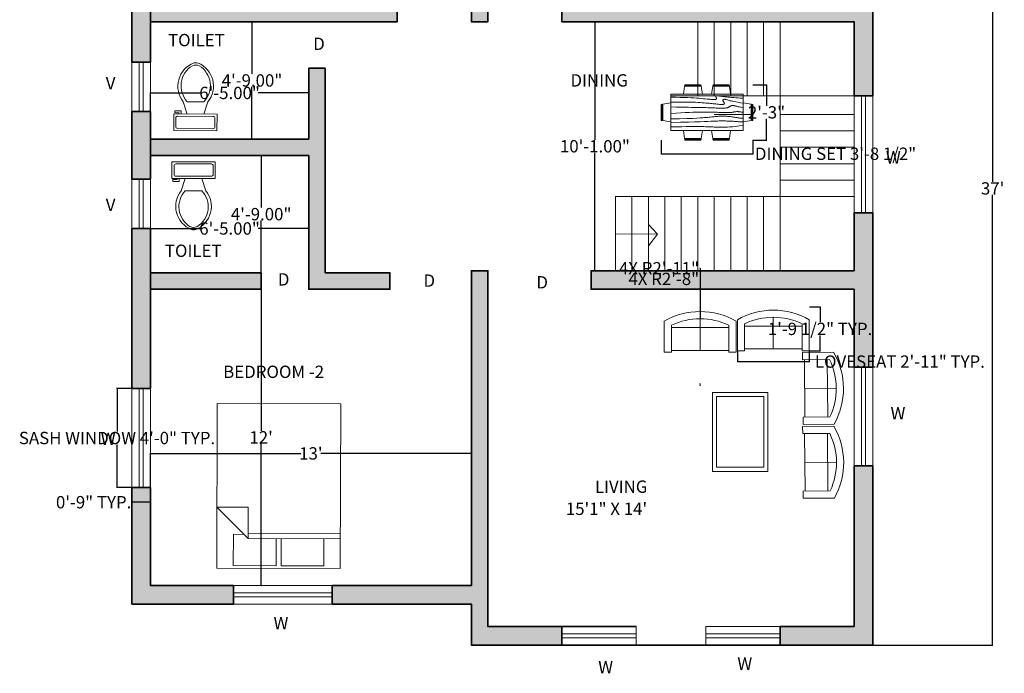
# Model space of a CAD drawing. Units: inches. Extents: x -977 to 1065, y -406 to 125.
# Tile 3 of 4: x 571 to 1049, y -406 to -89. Entities that reach past the tile are written whole.
import ezdxf

# ---------------------------------------------------------------- set-up
doc = ezdxf.new("R2010")
doc.units = ezdxf.units.IN
doc.header["$MEASUREMENT"] = 0
for name, color, linetype, lineweight in [('A-ANNO-DIMS', 2, 'Continuous', 13), ('A-ANNO-TEXT', 7, 'Continuous', 18), ('A-AREA-IDEN', 7, 'Continuous', 18), ('A-FLOR-FIXT', 8, 'Continuous', 18), ('A-FLOR-STRS', 7, 'Continuous', 18), ('A-FURN', 8, 'Continuous', 18), ('A-GLAZ', 5, 'Continuous', 18), ('A-WALL', 7, 'Continuous', 35), ('A-WALL-PATT', 252, 'Continuous', 13)]:
    doc.layers.add(name, color=color, linetype=linetype, lineweight=lineweight)
doc.styles.get("Standard").update_dxf_attribs({"font": 'arial.ttf'})
doc.dimstyles.get("Standard").update_dxf_attribs({"dimtxt": 6, "dimasz": 0.18, "dimexe": 0.18, "dimexo": 0.0625, "dimgap": 0.09, "dimtad": 0, "dimtih": 1, "dimtoh": 1, "dimzin": 0, "dimdsep": 46, "dimlunit": 3, "dimtxsty": 'Standard', "dimcen": 0.09, "dimadec": 0, "dimazin": 0, "dimtfac": 1, "dimtofl": 0, "dimtmove": 0, "dimatfit": 3, "dimfxl": 1, "dimtolj": 1, "dimtzin": 0, "dimarcsym": 0})

# ---------------------------------------------------------------- blocks, each defined once
blk = doc.blocks.new('Sofa - Roundback Loveseat 5 ft.')
for p, q in [((0, -32.44198), (0, -5.99998)), ((-24, -33.99998), (-24, -11.46958)), ((-23.9998, -13.38178), (23.99986, -13.38178)), ((24.00004, -33.99998), (24.00004, -11.46958)), ((-24, -32.44198), (24.00004, -32.44198))]:
    blk.add_line(p, q)
for points in [[(-24, -33.99998), (-30, -33.99998), (-30, -7.99998)], [(30.00004, -7.99998), (30.00004, -33.99998), (24.00004, -33.99998)]]:
    blk.add_lwpolyline(points)
for centre, radius, start, end in [((0, -60.24998), 60.24998, 60.13715, 119.8628), ((0, -61.38438), 55.38444, 64.32083, 115.6792)]:
    blk.add_arc(centre, radius, start, end)
blk = doc.blocks.new('*U27')
for p, q in [((9.5, -6), (9.5, -2)), ((-10, -8.5), (-8, -8.5)), ((-10, -9.5), (-10, -8.5)), ((-7, -9.5), (-10, -9.5)), ((-8, -8.5), (-8, -8)), ((-7, -8), (-7, -9.5)), ((-4, -8), (-6, -14)), ((4, -8), (6, -14)), ((4, -14), (-4, -14))]:
    blk.add_line(p, q)
blk.add_lwpolyline([(10.5, -8), (10.5, 0), (-10.5, 0), (-10.5, -8)], close=True)
for points in [[(-9.5, -2), (-9.5, -6)], [(8.5, -1), (-8.5, -1)], [(-8.5, -7), (8.5, -7)]]:
    blk.add_lwpolyline(points)
for centre, radius, start, end in [((-8.62, -1.88), 0.884, 81.8699, 188.1301), ((8.62, -1.88), 0.884, 351.8699, 98.1301), ((-8.62, -6.12), 0.884, 171.8699, 278.1301), ((8.62, -6.12), 0.884, 261.8699, 8.1301), ((3.52, -21.58), 12.17, 141.4691, 247.9714), ((4.2, -21.82), 11.33, 136.3677, 238.9468), ((-3.52, -21.58), 12.17, 292.0284, 38.5307), ((-4.2, -21.82), 11.33, 301.053, 43.6321), ((0, -27.88), 4, 245.7318, 294.2682), ((0, -29), 4, 254.8605, 285.1395)]:
    blk.add_arc(centre, radius, start, end)
blk = doc.blocks.new('Dining Set - 36 x 72 in.')
for p, q in [((-22.2343, 26.00059), (-23.4847, 17.99762)), ((-22.2304, 26), (-5.7608, 26)), ((-22, 27.5), (-22.1562, 26.50042)), ((-5.8416, 26.5), (-22.1534, 26.5)), ((-22, 27.5), (-6, 27.5)), ((-5.8437, 26.49966), (-6, 27.5)), ((-4.5152, 17.99762), (-5.7655, 25.99926)), ((5.7657, 26.00059), (4.5153, 17.99762)), ((5.7696, 26), (22.2392, 26)), ((6, 27.5), (5.8438, 26.50042)), ((22.1584, 26.5), (5.8466, 26.5)), ((6, 27.5), (22, 27.5)), ((22.1563, 26.49966), (22, 27.5)), ((23.4848, 17.99762), (22.2345, 25.99926)), ((36, 18), (-36, 18)), ((-36, 18), (-36, -18)), ((36, -18), (36, 18)), ((-45.5, 8), (-44.5004, 8.15617)), ((-45.5, 8), (-45.5, -8)), ((-44.5, -8.15843), (-44.5, 8.15338)), ((-44.0006, 8.23428), (-35.9976, 9.48474)), ((-44, 8.23041), (-44, -8.23915)), ((44.0006, 8.23428), (35.9976, 9.48474)), ((44, 8.23041), (44, -8.23915)), ((44.5, -8.15843), (44.5, 8.15338)), ((45.5, 8), (44.5005, 8.15617)), ((45.5, 8), (45.5, -8)), ((-44.4997, -8.15631), (-45.5, -8)), ((-35.9976, -9.48476), (-43.9993, -8.2345)), ((35.9976, -9.48476), (43.9993, -8.2345)), ((44.4997, -8.15631), (45.5, -8)), ((-36, -18), (36, -18)), ((-22.2343, -26.0006), (-23.4847, -17.99762)), ((-4.5152, -17.99762), (-5.7655, -25.99928)), ((5.7657, -26.0006), (4.5153, -17.99762)), ((23.4848, -17.99762), (22.2345, -25.99928)), ((-22.2304, -26), (-5.7608, -26)), ((-22, -27.5), (-22.1562, -26.50044)), ((-5.8416, -26.5), (-22.1534, -26.5)), ((-22, -27.5), (-6, -27.5)), ((-5.8437, -26.49967), (-6, -27.5)), ((5.7696, -26), (22.2392, -26)), ((6, -27.5), (5.8438, -26.50044)), ((22.1584, -26.5), (5.8466, -26.5)), ((6, -27.5), (22, -27.5)), ((22.1563, -26.49967), (22, -27.5))]:
    blk.add_line(p, q)
for points in [[(-36, 15), (-31.1772, 14.97754), (-26.8079, 14.91406), (-22.8538, 14.81543), (-19.276, 14.6875), (-16.0362, 14.53613), (-13.0957, 14.36718), (-10.4159, 14.18652), (-7.9583, 14), (-5.6904, 13.81315), (-3.6035, 13.63021), (-1.6954, 13.45508), (0.0365, 13.29166), (1.5945, 13.14388), (2.9811, 13.01562), (4.1988, 12.9108), (5.25, 12.83333), (6.1393, 12.78613), (6.8802, 12.76823), (7.4883, 12.77767), (7.9792, 12.8125), (8.3685, 12.87077), (8.6719, 12.95052), (8.9049, 13.0498), (9.0833, 13.16666), (9.2205, 13.29899), (9.3216, 13.44401), (9.3895, 13.59879), (9.4271, 13.76041), (9.4373, 13.92594), (9.4232, 14.09245), (9.3875, 14.257), (9.3333, 14.41666), (9.2638, 14.56917), (9.1836, 14.71484), (9.0975, 14.85465), (9.0104, 14.98958), (8.9272, 15.1206), (8.8529, 15.2487), (8.7922, 15.37483), (8.75, 15.5), (8.7305, 15.62467), (8.7344, 15.74739), (8.7617, 15.86621), (8.8125, 15.97916), (8.8867, 16.08431), (8.9844, 16.17968), (9.1055, 16.26334), (9.25, 16.33333), (9.4189, 16.38802), (9.6172, 16.42708), (9.8506, 16.45052), (10.125, 16.45833), (10.4463, 16.45052), (10.8203, 16.42708), (11.2529, 16.38802), (11.75, 16.33333), (12.3184, 16.26318), (12.9694, 16.17838), (13.7151, 16.07991), (14.5677, 15.96875), (15.5395, 15.84586), (16.6426, 15.71224), (17.8893, 15.56884), (19.2917, 15.41666), (20.859, 15.25667), (22.5879, 15.08984), (24.4721, 14.91715), (26.5052, 14.73958), (28.6809, 14.5581), (30.9929, 14.3737), (33.4347, 14.18733), (36, 14)], [(-36, 10), (-28.9766, 10.14274), (-23.1725, 10.20442), (-18.4241, 10.19775), (-14.5677, 10.13541), (-11.4399, 10.03011), (-8.877, 9.89453), (-6.7154, 9.74137), (-4.7917, 9.58333), (-2.9698, 9.43082), (-1.2246, 9.28515), (0.4415, 9.14534), (2.026, 9.01041), (3.5266, 8.87939), (4.9408, 8.7513), (6.266, 8.62516), (7.5, 8.5), (8.6411, 8.37549), (9.6914, 8.2539), (10.6538, 8.13818), (11.5312, 8.03125), (12.3267, 7.93603), (13.043, 7.85547), (13.6831, 7.79248), (14.25, 7.75), (14.7471, 7.7303), (15.1797, 7.73307), (15.5537, 7.75732), (15.875, 7.80208), (16.1494, 7.86637), (16.3828, 7.94922), (16.5811, 8.04964), (16.75, 8.16666), (16.8944, 8.29915), (17.0143, 8.44531), (17.1089, 8.60319), (17.1771, 8.77083), (17.218, 8.94629), (17.2305, 9.1276), (17.2137, 9.31282), (17.1667, 9.5), (17.0895, 9.6875), (16.987, 9.875), (16.8649, 10.0625), (16.7292, 10.25), (16.5856, 10.4375), (16.4401, 10.625), (16.2985, 10.8125), (16.1667, 11), (16.05, 11.18733), (15.9518, 11.3737), (15.8752, 11.5581), (15.8229, 11.73958), (15.798, 11.91715), (15.8034, 12.08984), (15.842, 12.25667), (15.9167, 12.41666), (16.0295, 12.56836), (16.1784, 12.70833), (16.3605, 12.83268), (16.5729, 12.9375), (16.8127, 13.01888), (17.0768, 13.07291), (17.3625, 13.0957), (17.6667, 13.08333), (17.9894, 13.03312), (18.3418, 12.94726), (18.7382, 12.82918), (19.1927, 12.68229), (19.7195, 12.51001), (20.3327, 12.31575), (21.0465, 12.10294), (21.875, 11.875), (22.8357, 11.63354), (23.959, 11.37304), (25.2786, 11.08618), (26.8282, 10.76562), (28.6414, 10.40405), (30.752, 9.99414), (33.1936, 9.52856), (36, 9)], [(-36, 5.5), (-30.7157, 5.3348), (-26.069, 5.20963), (-21.9946, 5.11767), (-18.4271, 5.05208), (-15.3009, 5.00602), (-12.5508, 4.97265), (-10.1112, 4.94515), (-7.9167, 4.91666), (-5.909, 4.88167), (-4.0586, 4.83984), (-2.3429, 4.79215), (-0.7396, 4.73958), (0.7739, 4.6831), (2.22, 4.6237), (3.6213, 4.56233), (5, 4.5), (6.373, 4.43782), (7.7344, 4.3776), (9.0723, 4.32129), (10.375, 4.27083), (11.6309, 4.22819), (12.8281, 4.19531), (13.9551, 4.17415), (15, 4.16666), (15.954, 4.17448), (16.819, 4.19791), (17.6001, 4.23698), (18.3021, 4.29166), (18.9299, 4.36198), (19.4883, 4.44791), (19.9823, 4.54948), (20.4167, 4.66666), (20.7969, 4.79899), (21.1302, 4.94401), (21.4245, 5.09879), (21.6875, 5.26041), (21.9271, 5.42594), (22.1511, 5.59245), (22.3672, 5.757), (22.5834, 5.91666), (22.8065, 6.06868), (23.0404, 6.21093), (23.2879, 6.34147), (23.5521, 6.45833), (23.8358, 6.55957), (24.142, 6.64323), (24.4735, 6.70735), (24.8334, 6.75), (25.2235, 6.76969), (25.642, 6.76692), (26.0858, 6.74267), (26.5521, 6.69791), (27.0379, 6.63362), (27.5404, 6.55078), (28.0565, 6.45036), (28.5834, 6.33333), (29.1242, 6.19987), (29.7071, 6.04687), (30.3661, 5.87044), (31.1354, 5.66666), (32.0493, 5.43164), (33.142, 5.16146), (34.4475, 4.85221), (36, 4.5)], [(-36, -1), (-30.7915, -0.6591), (-26.0195, -0.38216), (-21.6519, -0.16284), (-17.6563, 0.00521), (-14.0005, 0.12833), (-10.6523, 0.21289), (-7.5796, 0.26522), (-4.75, 0.29166), (-2.134, 0.29793), (0.2878, 0.28711), (2.5317, 0.26163), (4.6146, 0.22396), (6.5529, 0.17651), (8.3633, 0.12174), (10.0623, 0.06209), (11.6667, 0), (13.1899, -0.06201), (14.6341, -0.1211), (15.9982, -0.17432), (17.2813, -0.21875), (18.4823, -0.25147), (19.6003, -0.26953), (20.6343, -0.27002), (21.5834, -0.25), (22.4481, -0.20768), (23.2357, -0.14584), (23.9549, -0.06836), (24.6146, 0.02083), (25.2235, 0.11784), (25.7904, 0.21875), (26.3241, 0.31966), (26.8334, 0.41666), (27.3265, 0.50618), (27.8099, 0.58593), (28.2894, 0.65397), (28.7709, 0.70833), (29.2601, 0.74707), (29.763, 0.76823), (30.2855, 0.76985), (30.8334, 0.75), (31.4088, 0.70784), (31.9994, 0.64713), (32.589, 0.57275), (33.1615, 0.48958), (33.7008, 0.4025), (34.1908, 0.3164), (34.6153, 0.23616), (34.9584, 0.16666), (35.2099, 0.11165), (35.3848, 0.07031), (35.504, 0.04069), (35.5886, 0.02083), (35.6594, 0.00879), (35.7377, 0.0026), (35.8442, 0.00032), (36, 0)], [(-36, -6.5), (-27.1843, -6.31267), (-20.084, -6.1263), (-14.469, -5.9419), (-10.1094, -5.76042), (-6.7752, -5.58285), (-4.2363, -5.41016), (-2.2629, -5.24333), (-0.625, -5.08334), (0.8708, -4.93099), (2.2715, -4.78646), (3.5872, -4.64974), (4.8281, -4.52084), (6.0046, -4.39974), (7.127, -4.28646), (8.2053, -4.18099), (9.25, -4.08334), (10.2705, -3.99382), (11.2734, -3.91407), (12.2647, -3.84603), (13.25, -3.79167), (14.2354, -3.75293), (15.2266, -3.73177), (16.2295, -3.73015), (17.25, -3.75), (18.2912, -3.79248), (19.3451, -3.85547), (20.4009, -3.93604), (21.4479, -4.03125), (22.4754, -4.13819), (23.4727, -4.25391), (24.4289, -4.37549), (25.3334, -4.5), (26.1785, -4.62492), (26.9694, -4.74935), (27.7145, -4.87281), (28.4219, -4.99479), (29.1, -5.11483), (29.7572, -5.23242), (30.4016, -5.34709), (31.0417, -5.45834), (31.6837, -5.56437), (32.3262, -5.65821), (32.9658, -5.73153), (33.599, -5.77604), (34.2224, -5.78345), (34.8327, -5.74545), (35.4264, -5.65373), (36, -5.5)], [(-36, -10), (-26.4022, -9.81299), (-18.4675, -9.62891), (-11.9839, -9.45069), (-6.7396, -9.28125), (-2.5226, -9.12354), (0.8789, -8.98047), (3.6769, -8.85498), (6.0833, -8.75), (8.2767, -8.66765), (10.3021, -8.60677), (12.1712, -8.56543), (13.8958, -8.54167), (15.4876, -8.53353), (16.9583, -8.53907), (18.3197, -8.55632), (19.5834, -8.58334), (20.7616, -8.61841), (21.8685, -8.66081), (22.9188, -8.71004), (23.9271, -8.76563), (24.9081, -8.82707), (25.8763, -8.89388), (26.8465, -8.96558), (27.8334, -9.04167), (28.8474, -9.12118), (29.8828, -9.20117), (30.93, -9.27824), (31.9792, -9.34896), (33.0205, -9.40991), (34.0443, -9.45768), (35.0407, -9.48885), (36, -9.5)], [(-36, -14.5), (-30.0881, -14.33513), (-25.0332, -14.21224), (-20.7312, -14.12647), (-17.0781, -14.07292), (-13.97, -14.04671), (-11.3027, -14.04297), (-8.9724, -14.05681), (-6.875, -14.08334), (-4.9224, -14.11833), (-3.0905, -14.16016), (-1.3709, -14.20785), (0.2448, -14.26042), (1.7647, -14.3169), (3.1973, -14.3763), (4.5507, -14.43767), (5.8333, -14.5), (7.0554, -14.5621), (8.235, -14.62175), (9.3922, -14.67652), (10.5469, -14.72396), (11.7192, -14.76164), (12.929, -14.78711), (14.1965, -14.79794), (15.5417, -14.79167), (16.9933, -14.76424), (18.6152, -14.70508), (20.4804, -14.60197), (22.6615, -14.44271), (25.2312, -14.21509), (28.2624, -13.9069), (31.8277, -13.50594), (36, -13)]]:
    blk.add_lwpolyline(points)
blk = doc.blocks.new('Bed - Queen')
for p, q in [((0, -80.00003), (0, 0)), ((0, 0), (59.99999, 0)), ((59.99999, 0), (59.99999, -80.00003)), ((7.99999, -1.2), (28.79998, -1.2)), ((7.99999, -14.4), (7.99999, -1.2)), ((28.79998, -1.2), (28.79998, -14.4)), ((31.19999, -1.2), (51.99999, -1.2)), ((31.19999, -14.4), (31.19999, -1.2)), ((51.99999, -1.2), (51.99999, -16.4)), ((0, -14.4), (44.8, -14.4)), ((44.8, -16.8), (0, -16.8)), ((59.99999, -29.6), (44.8, -14.4)), ((44.8, -14.4), (44.8, -29.6)), ((51.99999, -16.4), (46.79936, -16.4)), ((44.8, -29.6), (59.99999, -29.6)), ((59.99999, -80.00003), (0, -80.00003))]:
    blk.add_line(p, q)
blk = doc.blocks.new('*D32')
at = {"layer": 'A-ANNO-DIMS', "color": 0, "lineweight": -2, "transparency": 16777216}
for p, q in [((985.15, 51.33), (1043.56, 51.33)), ((1043.38, 51.15), (1043.38, -167.51)), ((1043.38, -392.49), (1043.38, -173.82)), ((985.15, -392.67), (1043.56, -392.67))]:
    blk.add_line(p, q, dxfattribs=at)
at = {"layer": 'A-ANNO-DIMS', "color": 0, "transparency": 16777216}
for points in [[(1043.35, 51.15), (1043.41, 51.15), (1043.38, 51.33)], [(1043.35, -392.49), (1043.41, -392.49), (1043.38, -392.67)]]:
    blk.add_solid(points, dxfattribs=at)
at = {"layer": 'Defpoints', "color": 0, "transparency": 16777216}
for p in [(985.09, 51.33), (985.09, -392.67), (1043.38, -392.67)]:
    blk.add_point(p, dxfattribs=at)
at = {"layer": 'A-ANNO-DIMS', "color": 0, "transparency": 16777216, "insert": (1043.38, -170.67), "char_height": 6, "attachment_point": 5}
blk.add_mtext("\\A1;37'", dxfattribs=at)
blk = doc.blocks.new('*D35')
at = {"layer": 'A-ANNO-DIMS', "color": 0, "lineweight": -2, "transparency": 16777216}
for p, q in [((681.54, -89.67), (683.66, -89.67)), ((683.48, -89.85), (683.48, -115.01)), ((683.48, -146.49), (683.48, -121.32)), ((681.54, -146.67), (683.66, -146.67))]:
    blk.add_line(p, q, dxfattribs=at)
at = {"layer": 'A-ANNO-DIMS', "color": 0, "transparency": 16777216}
for points in [[(683.45, -89.85), (683.51, -89.85), (683.48, -89.67)], [(683.45, -146.49), (683.51, -146.49), (683.48, -146.67)]]:
    blk.add_solid(points, dxfattribs=at)
at = {"layer": 'Defpoints', "color": 0, "transparency": 16777216}
for p in [(681.48, -89.67), (681.48, -146.67), (683.48, -146.67)]:
    blk.add_point(p, dxfattribs=at)
at = {"layer": 'A-ANNO-DIMS', "color": 0, "transparency": 16777216, "insert": (683.48, -118.17), "char_height": 6, "attachment_point": 5}
blk.add_mtext('\\A1;4\'-9.00"', dxfattribs=at)
blk = doc.blocks.new('*D36')
at = {"layer": 'A-ANNO-DIMS', "color": 0, "lineweight": -2, "transparency": 16777216}
for p, q in [((634.09, -139.91), (634.09, -124.07)), ((634.27, -124.25), (658.68, -124.25)), ((710.91, -124.25), (686.5, -124.25)), ((711.09, -139.91), (711.09, -124.07))]:
    blk.add_line(p, q, dxfattribs=at)
at = {"layer": 'A-ANNO-DIMS', "color": 0, "transparency": 16777216}
for points in [[(634.27, -124.22), (634.27, -124.28), (634.09, -124.25)], [(710.91, -124.22), (710.91, -124.28), (711.09, -124.25)]]:
    blk.add_solid(points, dxfattribs=at)
at = {"layer": 'Defpoints', "color": 0, "transparency": 16777216}
for p in [(711.09, -124.25), (634.09, -139.97), (711.09, -139.97)]:
    blk.add_point(p, dxfattribs=at)
at = {"layer": 'A-ANNO-DIMS', "color": 0, "transparency": 16777216, "insert": (672.59, -124.25), "char_height": 6, "attachment_point": 5}
blk.add_mtext('\\A1;6\'-5.00"', dxfattribs=at)
blk = doc.blocks.new('*D41')
at = {"layer": 'A-ANNO-DIMS', "color": 0, "lineweight": -2, "transparency": 16777216}
for p, q in [((872.64, -89.67), (849.94, -89.67)), ((850.12, -89.85), (850.12, -147.01)), ((850.12, -210.49), (850.12, -153.32)), ((876.03, -210.67), (849.94, -210.67))]:
    blk.add_line(p, q, dxfattribs=at)
at = {"layer": 'A-ANNO-DIMS', "color": 0, "transparency": 16777216}
for points in [[(850.09, -89.85), (850.15, -89.85), (850.12, -89.67)], [(850.09, -210.49), (850.15, -210.49), (850.12, -210.67)]]:
    blk.add_solid(points, dxfattribs=at)
at = {"layer": 'Defpoints', "color": 0, "transparency": 16777216}
for p in [(872.7, -89.67), (850.12, -210.67), (876.09, -210.67)]:
    blk.add_point(p, dxfattribs=at)
at = {"layer": 'A-ANNO-DIMS', "color": 0, "transparency": 16777216, "insert": (850.12, -150.17), "char_height": 6, "attachment_point": 5}
blk.add_mtext('\\A1;10\'-1.00"', dxfattribs=at)
blk = doc.blocks.new('*D42')
at = {"layer": 'A-ANNO-DIMS', "color": 0, "lineweight": -2, "transparency": 16777216}
for p, q in [((634.09, -190.07), (634.09, -189.95)), ((634.27, -190.13), (658.68, -190.13)), ((710.91, -190.13), (686.5, -190.13)), ((711.09, -190.07), (711.09, -189.95))]:
    blk.add_line(p, q, dxfattribs=at)
at = {"layer": 'A-ANNO-DIMS', "color": 0, "transparency": 16777216}
for points in [[(634.27, -190.1), (634.27, -190.16), (634.09, -190.13)], [(710.91, -190.1), (710.91, -190.16), (711.09, -190.13)]]:
    blk.add_solid(points, dxfattribs=at)
at = {"layer": 'Defpoints', "color": 0, "transparency": 16777216}
for p in [(634.09, -190.13), (711.09, -190.13), (711.09, -190.13)]:
    blk.add_point(p, dxfattribs=at)
at = {"layer": 'A-ANNO-DIMS', "color": 0, "transparency": 16777216, "insert": (672.59, -190.13), "char_height": 6, "attachment_point": 5}
blk.add_mtext('\\A1;6\'-5.00"', dxfattribs=at)
blk = doc.blocks.new('*D43')
at = {"layer": 'A-ANNO-DIMS', "color": 0, "lineweight": -2, "transparency": 16777216}
for p, q in [((687.92, -154.85), (687.92, -180.01)), ((687.99, -154.67), (688.1, -154.67)), ((687.92, -211.49), (687.92, -186.32)), ((687.99, -211.67), (688.1, -211.67))]:
    blk.add_line(p, q, dxfattribs=at)
at = {"layer": 'A-ANNO-DIMS', "color": 0, "transparency": 16777216}
for points in [[(687.89, -154.85), (687.95, -154.85), (687.92, -154.67)], [(687.89, -211.49), (687.95, -211.49), (687.92, -211.67)]]:
    blk.add_solid(points, dxfattribs=at)
at = {"layer": 'Defpoints', "color": 0, "transparency": 16777216}
for p in [(687.92, -154.67), (687.92, -154.67), (687.92, -211.67)]:
    blk.add_point(p, dxfattribs=at)
at = {"layer": 'A-ANNO-DIMS', "color": 0, "transparency": 16777216, "insert": (687.92, -183.17), "char_height": 6, "attachment_point": 5}
blk.add_mtext('\\A1;4\'-9.00"', dxfattribs=at)
blk = doc.blocks.new('*D44')
at = {"layer": 'A-ANNO-DIMS', "color": 0, "lineweight": -2, "transparency": 16777216}
for p, q in [((687.92, -219.85), (687.92, -288.56)), ((687.99, -219.67), (688.1, -219.67)), ((687.92, -363.49), (687.92, -294.77)), ((687.99, -363.67), (688.1, -363.67))]:
    blk.add_line(p, q, dxfattribs=at)
at = {"layer": 'A-ANNO-DIMS', "color": 0, "transparency": 16777216}
for points in [[(687.89, -219.85), (687.95, -219.85), (687.92, -219.67)], [(687.89, -363.49), (687.95, -363.49), (687.92, -363.67)]]:
    blk.add_solid(points, dxfattribs=at)
at = {"layer": 'Defpoints', "color": 0, "transparency": 16777216}
for p in [(687.92, -219.67), (687.92, -363.67), (687.92, -363.67)]:
    blk.add_point(p, dxfattribs=at)
at = {"layer": 'A-ANNO-DIMS', "color": 0, "transparency": 16777216, "insert": (687.92, -291.67), "char_height": 6, "attachment_point": 5}
blk.add_mtext("\\A1;12'", dxfattribs=at)
blk = doc.blocks.new('*D45')
at = {"layer": 'A-ANNO-DIMS', "color": 0, "lineweight": -2, "transparency": 16777216}
for p, q in [((634.09, -315.92), (634.09, -299.29)), ((634.27, -299.47), (707.19, -299.47)), ((789.91, -299.47), (716.99, -299.47)), ((790.09, -315.92), (790.09, -299.29))]:
    blk.add_line(p, q, dxfattribs=at)
at = {"layer": 'A-ANNO-DIMS', "color": 0, "transparency": 16777216}
for points in [[(634.27, -299.44), (634.27, -299.5), (634.09, -299.47)], [(789.91, -299.44), (789.91, -299.5), (790.09, -299.47)]]:
    blk.add_solid(points, dxfattribs=at)
at = {"layer": 'Defpoints', "color": 0, "transparency": 16777216}
for p in [(790.09, -299.47), (634.09, -315.98), (790.09, -315.98)]:
    blk.add_point(p, dxfattribs=at)
at = {"layer": 'A-ANNO-DIMS', "color": 0, "transparency": 16777216, "insert": (712.09, -299.47), "char_height": 6, "attachment_point": 5}
blk.add_mtext("\\A1;13'", dxfattribs=at)
blk = doc.blocks.new('WIN-48-SASH')
for p, q in [((48, 9), (0, 9)), ((48, 5.5), (0, 5.5)), ((0, 3.5), (48, 3.5)), ((0, 0), (48, 0))]:
    blk.add_line(p, q)
for points in [[(48, 9), (0, 9)], [(48, 0), (0, 0)]]:
    blk.add_lwpolyline(points)
blk = doc.blocks.new('WIN-24-SASH')
for p, q in [((0, 5.5), (24, 5.5)), ((24, 9), (24, 0)), ((24, 3.5), (0, 3.5)), ((24, 0), (0, 0))]:
    blk.add_line(p, q)
for points in [[(0, 9), (24, 9)], [(0, 0), (24, 0)]]:
    blk.add_lwpolyline(points)
blk = doc.blocks.new('*D54')
at = {"layer": 'A-ANNO-DIMS', "color": 0, "lineweight": -2, "transparency": 16777216}
for p, q in [((919.36, -249.67), (919.36, -255.02)), ((954.28, -249.67), (954.28, -255.02)), ((919.54, -254.84), (954.1, -254.84)), ((954.28, -254.84), (954.46, -254.84))]:
    blk.add_line(p, q, dxfattribs=at)
at = {"layer": 'A-ANNO-DIMS', "color": 0, "transparency": 16777216}
for points in [[(919.54, -254.81), (919.54, -254.87), (919.36, -254.84)], [(954.1, -254.81), (954.1, -254.87), (954.28, -254.84)]]:
    blk.add_solid(points, dxfattribs=at)
at = {"layer": 'Defpoints', "color": 0, "transparency": 16777216}
for p in [(919.36, -249.61), (954.28, -249.61), (954.28, -254.84)]:
    blk.add_point(p, dxfattribs=at)
at = {"layer": 'A-ANNO-DIMS', "color": 0, "transparency": 16777216, "insert": (998.32, -254.84), "char_height": 6, "attachment_point": 5}
blk.add_mtext('\\A1;LOVESEAT 2\'-11" TYP.', dxfattribs=at)
blk = doc.blocks.new('*D55')
at = {"layer": 'A-ANNO-DIMS', "color": 0, "lineweight": -2, "transparency": 16777216}
for p, q in [((954.34, -228.27), (959.69, -228.27)), ((959.51, -228.45), (959.51, -235.74)), ((959.51, -249.43), (959.51, -242.13)), ((954.34, -249.61), (959.69, -249.61))]:
    blk.add_line(p, q, dxfattribs=at)
at = {"layer": 'A-ANNO-DIMS', "color": 0, "transparency": 16777216}
for points in [[(959.48, -228.45), (959.54, -228.45), (959.51, -228.27)], [(959.48, -249.43), (959.54, -249.43), (959.51, -249.61)]]:
    blk.add_solid(points, dxfattribs=at)
at = {"layer": 'Defpoints', "color": 0, "transparency": 16777216}
for p in [(954.28, -228.27), (959.51, -228.27), (954.28, -249.61)]:
    blk.add_point(p, dxfattribs=at)
at = {"layer": 'A-ANNO-DIMS', "color": 0, "transparency": 16777216, "insert": (959.51, -238.94), "char_height": 6, "attachment_point": 5}
blk.add_mtext('\\A1;1\'-9 1/2" TYP.', dxfattribs=at)
blk = doc.blocks.new('*D56')
at = {"layer": 'A-ANNO-DIMS', "color": 0, "lineweight": -2, "transparency": 16777216}
for p, q in [((625.03, -267.98), (617.71, -267.98)), ((617.89, -268.16), (617.89, -288.79)), ((617.89, -315.8), (617.89, -295.18)), ((625.03, -315.98), (617.71, -315.98))]:
    blk.add_line(p, q, dxfattribs=at)
at = {"layer": 'A-ANNO-DIMS', "color": 0, "transparency": 16777216}
for points in [[(617.86, -268.16), (617.92, -268.16), (617.89, -267.98)], [(617.86, -315.8), (617.92, -315.8), (617.89, -315.98)]]:
    blk.add_solid(points, dxfattribs=at)
at = {"layer": 'Defpoints', "color": 0, "transparency": 16777216}
for p in [(617.89, -267.98), (625.09, -267.98), (625.09, -315.98)]:
    blk.add_point(p, dxfattribs=at)
at = {"layer": 'A-ANNO-DIMS', "color": 0, "transparency": 16777216, "insert": (617.89, -291.98), "char_height": 6, "attachment_point": 5}
blk.add_mtext('\\A1;SASH WINDOW 4\'-0" TYP.', dxfattribs=at)
blk = doc.blocks.new('*D57')
at = {"layer": 'A-ANNO-DIMS', "color": 0, "lineweight": -2, "transparency": 16777216}
for p, q in [((625.09, -316.04), (625.09, -323.36)), ((634.09, -316.04), (634.09, -323.36)), ((625.09, -323.18), (624.91, -323.18)), ((633.91, -323.18), (625.27, -323.18))]:
    blk.add_line(p, q, dxfattribs=at)
at = {"layer": 'A-ANNO-DIMS', "color": 0, "transparency": 16777216}
for points in [[(625.27, -323.15), (625.27, -323.21), (625.09, -323.18)], [(633.91, -323.15), (633.91, -323.21), (634.09, -323.18)]]:
    blk.add_solid(points, dxfattribs=at)
at = {"layer": 'Defpoints', "color": 0, "transparency": 16777216}
for p in [(625.09, -315.98), (634.09, -315.98), (625.09, -323.18)]:
    blk.add_point(p, dxfattribs=at)
at = {"layer": 'A-ANNO-DIMS', "color": 0, "transparency": 16777216, "insert": (606.53, -323.18), "char_height": 6, "attachment_point": 5}
blk.add_mtext('\\A1;0\'-9" TYP.', dxfattribs=at)
blk = doc.blocks.new('*D66')
at = {"layer": 'A-ANNO-DIMS', "color": 0, "lineweight": -2, "transparency": 16777216}
for p, q in [((882.35, -147.2), (882.35, -153.99)), ((926.83, -147.2), (926.83, -153.99)), ((882.53, -153.81), (926.65, -153.81)), ((926.83, -153.81), (927.01, -153.81))]:
    blk.add_line(p, q, dxfattribs=at)
at = {"layer": 'A-ANNO-DIMS', "color": 0, "transparency": 16777216}
for points in [[(882.53, -153.78), (882.53, -153.84), (882.35, -153.81)], [(926.65, -153.78), (926.65, -153.84), (926.83, -153.81)]]:
    blk.add_solid(points, dxfattribs=at)
at = {"layer": 'Defpoints', "color": 0, "transparency": 16777216}
for p in [(882.35, -147.14), (926.83, -147.14), (926.83, -153.81)]:
    blk.add_point(p, dxfattribs=at)
at = {"layer": 'A-ANNO-DIMS', "color": 0, "transparency": 16777216, "insert": (967.06, -153.81), "char_height": 6, "attachment_point": 5}
blk.add_mtext('\\A1;DINING SET 3\'-8 1/2"', dxfattribs=at)
blk = doc.blocks.new('*D67')
at = {"layer": 'A-ANNO-DIMS', "color": 0, "lineweight": -2, "transparency": 16777216}
for p, q in [((926.89, -120.26), (933.68, -120.26)), ((933.5, -120.44), (933.5, -130.54)), ((933.5, -146.96), (933.5, -136.85)), ((926.89, -147.14), (933.68, -147.14))]:
    blk.add_line(p, q, dxfattribs=at)
at = {"layer": 'A-ANNO-DIMS', "color": 0, "transparency": 16777216}
for points in [[(933.47, -120.44), (933.53, -120.44), (933.5, -120.26)], [(933.47, -146.96), (933.53, -146.96), (933.5, -147.14)]]:
    blk.add_solid(points, dxfattribs=at)
at = {"layer": 'Defpoints', "color": 0, "transparency": 16777216}
for p in [(926.83, -120.26), (933.5, -120.26), (926.83, -147.14)]:
    blk.add_point(p, dxfattribs=at)
at = {"layer": 'A-ANNO-DIMS', "color": 0, "transparency": 16777216, "insert": (933.5, -133.7), "char_height": 6, "attachment_point": 5}
blk.add_mtext('\\A1;2\'-3"', dxfattribs=at)
blk = doc.blocks.new('*D68')
at = {"layer": 'A-ANNO-DIMS', "color": 0, "lineweight": -2, "transparency": 16777216}
for p, q in [((901.09, -209.46), (901.27, -209.46)), ((901.27, -209.46), (901.27, -230.32)), ((901.18, -265.57), (901.36, -265.57)), ((901.27, -265.66), (901.27, -265.48))]:
    blk.add_line(p, q, dxfattribs=at)
at = {"layer": 'A-ANNO-DIMS', "color": 0, "transparency": 16777216}
blk.add_solid([(901.3, -230.32), (901.24, -230.32), (901.27, -230.5)], dxfattribs=at)
at = {"layer": 'Defpoints', "color": 0, "transparency": 16777216}
for p in [(901.27, -230.5), (901.27, -265.57)]:
    blk.add_point(p, dxfattribs=at)
at = {"layer": 'A-ANNO-DIMS', "color": 0, "transparency": 16777216, "insert": (881.26, -209.46), "char_height": 6, "attachment_point": 5}
blk.add_mtext('\\A1;4X R2\'-11"', dxfattribs=at)
blk = doc.blocks.new('*D69')
at = {"layer": 'A-ANNO-DIMS', "color": 0, "lineweight": -2, "transparency": 16777216}
for p, q in [((901.09, -214.65), (901.27, -214.65)), ((901.27, -214.65), (901.27, -233.81)), ((901.18, -266.23), (901.36, -266.23)), ((901.27, -266.32), (901.27, -266.14))]:
    blk.add_line(p, q, dxfattribs=at)
at = {"layer": 'A-ANNO-DIMS', "color": 0, "transparency": 16777216}
blk.add_solid([(901.3, -233.81), (901.24, -233.81), (901.27, -233.99)], dxfattribs=at)
at = {"layer": 'Defpoints', "color": 0, "transparency": 16777216}
for p in [(901.27, -233.99), (901.27, -266.23)]:
    blk.add_point(p, dxfattribs=at)
at = {"layer": 'A-ANNO-DIMS', "color": 0, "transparency": 16777216, "insert": (883.59, -214.65), "char_height": 6, "attachment_point": 5}
blk.add_mtext('\\A1;4X R2\'-8"', dxfattribs=at)

msp = doc.modelspace()

# ---------------------------------------------------------------- hatches: boundary and pattern name
at = {"layer": 'A-WALL-PATT'}
h = msp.add_hatch(color=256, dxfattribs=at)
h.dxf.hatch_style = 1
h.paths.add_polyline_path([(798.089, 42.333), (798.089, -89.667), (790.089, -89.667), (790.089, 42.333), (735.18, 42.333), (735.18, 51.333), (842.634, 51.333), (842.634, 42.333)])
h = msp.add_hatch(color=256, dxfattribs=at)
h.dxf.hatch_style = 1
h.paths.add_polyline_path([(985.089, -125.667), (985.089, -48.655), (976.089, -48.655), (976.089, -81.667), (834.089, -81.667), (834.089, -89.667), (976.089, -89.667), (976.089, -125.667)])
h = msp.add_hatch(color=256, dxfattribs=at)
h.dxf.hatch_style = 1
h.paths.add_polyline_path([(625.089, -109.279), (625.089, -60.85), (634.089, -60.85), (634.089, -109.279)])
h = msp.add_hatch(color=256, dxfattribs=at)
h.dxf.hatch_style = 1
h.paths.add_polyline_path([(754.089, -81.667), (634.089, -81.667), (634.089, -89.667), (754.089, -89.667)])
h = msp.add_hatch(color=256, dxfattribs=at)
h.dxf.hatch_style = 1
h.paths.add_polyline_path([(634.089, -154.667), (711.089, -154.667), (711.089, -219.667), (750.462, -219.667), (750.462, -211.667), (719.089, -211.667), (719.089, -112.271), (711.089, -112.271), (711.089, -146.667), (634.089, -146.667)])
h = msp.add_hatch(color=256, dxfattribs=at)
h.dxf.hatch_style = 1
h.paths.add_polyline_path([(625.089, -166.132), (625.089, -133.279), (634.089, -133.279), (634.089, -166.132)])
h = msp.add_hatch(color=256, dxfattribs=at)
h.dxf.hatch_style = 1
h.paths.add_polyline_path([(976.089, -210.667), (976.089, -182.506), (985.089, -182.506), (985.089, -257.573), (976.089, -257.573), (976.089, -219.667), (848.282, -219.667), (848.282, -210.667)])
h = msp.add_hatch(color=256, dxfattribs=at)
h.dxf.hatch_style = 1
h.paths.add_polyline_path([(634.089, -190.132), (634.089, -267.982), (625.089, -267.982), (625.089, -190.132)])
h = msp.add_hatch(color=256, dxfattribs=at)
h.dxf.hatch_style = 1
h.paths.add_polyline_path([(634.089, -190.132), (634.089, -267.982), (625.089, -267.982), (625.089, -190.132)])
edge = h.paths.add_edge_path()
edge.add_line((634.089, -219.667), (687.923, -219.667))
edge.add_line((634.089, -211.667), (687.923, -211.667))
edge.add_line((687.923, -211.667), (687.923, -219.667))
h = msp.add_hatch(color=256, dxfattribs=at)
h.dxf.hatch_style = 1
h.paths.add_polyline_path([(687.923, -219.667), (634.089, -219.667), (634.089, -211.667), (687.923, -211.667)])
h = msp.add_hatch(color=256, dxfattribs=at)
h.dxf.hatch_style = 1
h.paths.add_polyline_path([(834.089, -383.667), (834.089, -392.667), (790.089, -392.667), (790.089, -372.667), (722.517, -372.667), (722.517, -363.667), (790.089, -363.667), (790.089, -210.667), (798.089, -210.667), (798.089, -383.667)])
h = msp.add_hatch(color=256, dxfattribs=at)
h.dxf.hatch_style = 1
h.paths.add_polyline_path([(976.089, -305.573), (976.089, -383.667), (940.089, -383.667), (940.089, -392.667), (985.089, -392.667), (985.089, -305.573)])
h = msp.add_hatch(color=256, dxfattribs=at)
h.dxf.hatch_style = 1
h.paths.add_polyline_path([(674.517, -363.667), (634.089, -363.667), (634.089, -315.982), (625.089, -315.982), (625.089, -372.667), (674.517, -372.667)])

# ---------------------------------------------------------------- linework, layer by layer
at = {"layer": 'A-FLOR-STRS'}
for p, q in [((880.595, -192.851), (876.089, -188.143)), ((876.089, -188.143), (880.595, -192.851)), ((860.089, -192.667), (880.595, -192.851)), ((880.595, -192.851), (876.089, -198.645))]:
    msp.add_line(p, q, dxfattribs=at)
for points in [[(900.089, -89.667), (900.089, -125.667)], [(908.089, -89.667), (908.089, -125.667)], [(916.089, -89.667), (916.089, -125.667)], [(924.089, -89.667), (924.089, -125.667)], [(932.089, -89.667), (932.089, -125.667)], [(940.089, -89.667), (940.089, -210.667)], [(886.992, -125.667), (976.089, -125.667)], [(908.089, -134.667), (926.828, -134.667)], [(940.089, -134.667), (976.089, -134.667)], [(940.089, -142.667), (976.089, -142.667)], [(940.089, -150.667), (976.089, -150.667)], [(940.089, -158.667), (976.089, -158.667)], [(940.089, -166.667), (976.089, -166.667)], [(860.089, -174.667), (976.089, -174.667)], [(860.089, -174.667), (976.089, -174.667)], [(860.089, -174.667), (860.089, -210.667)], [(868.089, -174.667), (868.089, -210.667)], [(876.089, -174.667), (876.089, -210.667)], [(884.089, -174.667), (884.089, -210.667)], [(892.089, -174.667), (892.089, -210.667)], [(900.089, -174.667), (900.089, -210.667)], [(908.089, -174.667), (908.089, -210.667)], [(916.089, -174.667), (916.089, -210.667)], [(924.089, -174.667), (924.089, -210.667)], [(932.089, -174.667), (932.089, -210.667)]]:
    msp.add_lwpolyline(points, dxfattribs=at)
at = {"layer": 'A-FURN'}
for points in [[(907.266, -269.87), (934.166, -269.87), (934.166, -308.193), (907.266, -308.193)], [(909.266, -271.87), (932.166, -271.87), (932.166, -306.193), (909.266, -306.193)]]:
    msp.add_lwpolyline(points, close=True, dxfattribs=at)
at = {"layer": 'A-GLAZ'}
for p, q in [((634.089, -109.279), (634.089, -133.279)), ((976.089, -125.667), (976.089, -164.301)), ((979.589, -125.667), (979.589, -182.506)), ((981.589, -182.506), (981.589, -125.667)), ((985.089, -164.301), (985.089, -125.667)), ((625.089, -133.279), (634.089, -133.279)), ((634.089, -170.699), (634.089, -190.132)), ((976.089, -305.573), (985.089, -305.573)), ((834.089, -383.667), (870.089, -383.667)), ((834.089, -387.167), (870.089, -387.167)), ((870.089, -383.667), (870.089, -392.667)), ((904.089, -383.667), (904.089, -392.667)), ((834.089, -389.167), (870.089, -389.167)), ((904.089, -389.167), (940.089, -389.167)), ((834.089, -392.667), (870.089, -392.667)), ((849.891, -392.667), (849.891, -392.667)), ((904.089, -392.667), (940.089, -392.667))]:
    msp.add_line(p, q, dxfattribs=at)
for points in [[(976.089, -125.667), (976.089, -182.506)], [(985.089, -125.667), (985.089, -182.506)], [(940.089, -383.667), (904.089, -383.667)], [(940.089, -387.167), (904.089, -387.167)]]:
    msp.add_lwpolyline(points, dxfattribs=at)
at = {"layer": 'A-WALL'}
for points in [[(798.089, 42.333), (798.089, -89.667), (790.089, -89.667), (790.089, 42.333), (735.18, 42.333), (735.18, 51.333), (842.634, 51.333), (842.634, 42.333)], [(754.089, -81.667), (634.089, -81.667), (634.089, -89.667), (754.089, -89.667)], [(634.089, -154.667), (711.089, -154.667), (711.089, -219.667), (750.462, -219.667), (750.462, -211.667), (719.089, -211.667), (719.089, -112.271), (711.089, -112.271), (711.089, -146.667), (634.089, -146.667)], [(976.089, -210.667), (976.089, -182.506), (985.089, -182.506), (985.089, -257.573), (976.089, -257.573), (976.089, -219.667), (848.282, -219.667), (848.282, -210.667)], [(687.923, -219.667), (634.089, -219.667), (634.089, -211.667), (687.923, -211.667)], [(834.089, -383.667), (834.089, -392.667), (790.089, -392.667), (790.089, -372.667), (722.517, -372.667), (722.517, -363.667), (790.089, -363.667), (790.089, -210.667), (798.089, -210.667), (798.089, -383.667)], [(976.089, -305.573), (976.089, -383.667), (940.089, -383.667), (940.089, -392.667), (985.089, -392.667), (985.089, -305.573)], [(674.517, -363.667), (634.089, -363.667), (634.089, -315.982), (625.089, -315.982), (625.089, -372.667), (674.517, -372.667)]]:
    msp.add_lwpolyline(points, close=True, dxfattribs=at)
for points in [[(985.089, -125.667), (985.089, -48.655), (976.089, -48.655), (976.089, -81.667), (834.089, -81.667), (834.089, -89.667), (976.089, -89.667), (976.089, -125.667), (985.089, -125.667), (985.089, -116.301)], [(625.089, -109.279), (625.089, -60.85), (634.089, -60.85), (634.089, -81.667)], [(634.089, -89.667), (634.089, -109.279), (625.089, -109.279)], [(625.089, -166.132), (625.089, -133.279), (634.089, -133.279), (634.089, -146.667)], [(634.089, -154.667), (634.089, -166.132), (625.089, -166.132)], [(634.089, -219.667), (634.089, -267.982), (625.089, -267.982), (625.089, -190.132), (634.089, -190.132)], [(634.089, -190.132), (634.089, -211.667)], [(634.089, -219.667), (687.923, -219.667)], [(870.089, -383.667), (798.089, -383.667)], [(940.089, -392.667), (834.089, -392.667)]]:
    msp.add_lwpolyline(points, dxfattribs=at)

# ---------------------------------------------------------------- block references
at = {"layer": 'A-FLOR-FIXT', "xscale": -1, "rotation": 179.5018045392263}
msp.add_blockref('*U27', (655.934, -142.552), dxfattribs=at)
at = {"layer": 'A-FLOR-FIXT'}
msp.add_blockref('*U27', (655.08, -157.758), dxfattribs=at)
at = {"layer": 'A-FURN'}
for name, p, xscale, yscale, zscale in [('Dining Set - 36 x 72 in.', (904.588, -133.699), 0.4887798293897647, 0.4887798293897647, 0.4887798293897647), ('Sofa - Roundback Loveseat 5 ft.', (901.273, -230.502), 0.5819904717945719, 0.5819904717945719, 0.5819904717945719), ('Sofa - Roundback Loveseat 5 ft.', (936.816, -229.817), 0.5819904717945719, 0.5819904717945719, 0.5819904717945719)]:
    msp.add_blockref(name, p, dxfattribs=dict(at, xscale=xscale, yscale=yscale, zscale=zscale))
at = {"layer": 'A-FURN', "xscale": 0.5819904717945719, "yscale": 0.5819904717945719, "zscale": 0.5819904717945719, "rotation": 270.5074165948745}
for p in [(970.903, -267.705), (970.996, -303.642)]:
    msp.add_blockref('Sofa - Roundback Loveseat 5 ft.', p, dxfattribs=at)
at = {"layer": 'A-FURN', "rotation": 179.8323037866585}
msp.add_blockref('Bed - Queen', (726.378, -355.349), dxfattribs=at)
at = {"layer": 'A-GLAZ', "extrusion": (0, 0, -1), "zscale": -1, "rotation": 90.0000000000003}
msp.add_blockref('WIN-24-SASH', (-625.089, -133.279), dxfattribs=at)
at = {"layer": 'A-GLAZ'}
for name, p, rotation in [('WIN-24-SASH', (625.089, -166.132), 270.0000000000002), ('WIN-48-SASH', (976.089, -257.573), 269.9999999999999), ('WIN-48-SASH', (634.089, -315.982), 89.99999999999987), ('WIN-48-SASH', (722.517, -363.667), 180)]:
    msp.add_blockref(name, p, dxfattribs=dict(at, rotation=rotation))

# ---------------------------------------------------------------- texts
at = {"layer": 'A-ANNO-TEXT', "char_height": 6, "attachment_point": 1}
for s, insert in [('D ', (713.233, -97.355)), ('V ', (612.424, -116.533)), ('W ', (991.539, -152.549)), ('V ', (612.424, -175.657)), ('D ', (696.05, -211.872)), ('D ', (766.815, -212.486)), ('D ', (821.688, -213.303)), ('W ', (993.793, -276.978)), ('W ', (610.006, -289.44)), ('W ', (693.963, -378.961)), ('W ', (851.734, -400.356)), ('W ', (919.35, -398.667))]:
    msp.add_mtext_dynamic_manual_height_columns(s, width=77.77408, gutter_width=1, heights=[0], dxfattribs=dict(at, insert=insert))
at = {"layer": 'A-AREA-IDEN', "char_height": 6, "attachment_point": 1}
for s, heights, insert in [('TOILET ', [0], (642.686, -95.558)), ('DINING', [0], (838.237, -115.14)), ('TOILET ', [0], (641.145, -197.967)), ('BEDROOM -2', [0], (669.472, -256.805)), ('LIVING', [6.205], (850.118, -312.638)), ('15\'1" X 14\'', [0], (835.988, -323.393))]:
    msp.add_mtext_dynamic_manual_height_columns(s, width=77.77408, gutter_width=1, heights=heights, dxfattribs=dict(at, insert=insert))

# ---------------------------------------------------------------- dimensions: what is measured, and where the dimension line sits
at = {"layer": 'A-ANNO-DIMS'}
for base, p1, p2, override, picture, middle in [((1043.377, -392.667), (985.089, 51.333), (985.089, -392.667), {"dimclrd": 0, "dimclre": 0, "dimclrt": 0}, '*D32', (1043.377, -170.667)), ((683.483, -146.667), (681.475, -89.667), (681.475, -146.667), {"dimclrd": 0, "dimclre": 0, "dimclrt": 0}, '*D35', (683.483, -118.167)), ((850.12, -210.667), (872.702, -89.667), (876.089, -210.667), {"dimclrd": 0, "dimclre": 0, "dimclrt": 0}, '*D41', (850.12, -150.167)), ((933.5, -120.258), (926.828, -147.141), (926.828, -120.258), {"dimdec": 1, "dimlfac": 1, "dimrnd": 0, "dimzin": 1, "dimdsep": 46, "dimlunit": 4, "dimfrac": 2}, '*D67', (933.5, -133.699)), ((687.923, -154.667), (687.923, -211.667), (687.923, -154.667), {"dimclrd": 0, "dimclre": 0, "dimclrt": 0}, '*D43', (687.923, -183.167)), ((687.923, -363.667), (687.923, -219.667), (687.923, -363.667), {"dimclrd": 0, "dimclre": 0, "dimclrt": 0}, '*D44', (687.923, -291.667))]:
    dim = msp.add_linear_dim(base=base, p1=p1, p2=p2, angle=90, dimstyle='Standard', override=override, dxfattribs=at)
    dim.commit()
    dim.dimension.update_dxf_attribs({"geometry": picture, "text_midpoint": middle})
for base, p1, p2, picture, middle in [((711.089, -124.247), (634.089, -139.973), (711.089, -139.973), '*D36', (672.589, -124.247)), ((711.089, -190.132), (634.089, -190.132), (711.089, -190.132), '*D42', (672.589, -190.132)), ((790.089, -299.473), (634.089, -315.982), (790.089, -315.982), '*D45', (712.089, -299.473))]:
    dim = msp.add_linear_dim(base=base, p1=p1, p2=p2, dimstyle='Standard', override={"dimclrd": 0, "dimclre": 0, "dimclrt": 0}, dxfattribs=at)
    dim.commit()
    dim.dimension.update_dxf_attribs({"geometry": picture, "text_midpoint": middle})
for base, p1, p2, text, picture, middle in [((926.828, -153.813), (882.349, -147.141), (926.828, -147.141), 'DINING SET <>', '*D66', (967.062, -153.813)), ((954.276, -254.843), (919.357, -249.605), (954.276, -249.605), 'LOVESEAT <> TYP.', '*D54', (998.322, -254.843))]:
    dim = msp.add_linear_dim(base=base, p1=p1, p2=p2, text=text, dimstyle='Standard', override={"dimdec": 1, "dimlfac": 1, "dimrnd": 0, "dimzin": 1, "dimdsep": 46, "dimlunit": 4, "dimfrac": 2}, dxfattribs=at)
    dim.commit()
    dim.dimension.update_dxf_attribs({"geometry": picture, "text_midpoint": middle})
for center, mpoint, picture, middle in [((901.273, -265.567), (901.273, -230.502), '*D68', (881.259, -209.463)), ((901.273, -266.227), (901.273, -233.994), '*D69', (883.59, -214.654))]:
    dim = msp.add_radius_dim(center=center, mpoint=mpoint, text='4X <>', dimstyle='Standard', override={"dimdec": 1, "dimlfac": 1, "dimrnd": 0, "dimzin": 1, "dimdsep": 46, "dimlunit": 4, "dimfrac": 2}, dxfattribs=at)
    dim.commit()
    dim.dimension.update_dxf_attribs({"geometry": picture, "text_midpoint": middle, "dimtype": 164})
for base, p1, p2, angle, text, picture, middle in [((959.514, -228.265), (954.276, -249.605), (954.276, -228.265), 90, '<> TYP.', '*D55', (959.514, -238.935)), ((617.889, -267.982), (625.089, -315.982), (625.089, -267.982), 90, 'SASH WINDOW <> TYP.', '*D56', (617.889, -291.982)), ((625.089, -323.182), (634.089, -315.982), (625.089, -315.982), 180, '<> TYP.', '*D57', (606.532, -323.182))]:
    dim = msp.add_linear_dim(base=base, p1=p1, p2=p2, angle=angle, text=text, dimstyle='Standard', override={"dimdec": 1, "dimlfac": 1, "dimrnd": 0, "dimzin": 1, "dimdsep": 46, "dimlunit": 4, "dimfrac": 2}, dxfattribs=at)
    dim.commit()
    dim.dimension.update_dxf_attribs({"geometry": picture, "text_midpoint": middle})

doc.saveas('drawing.dxf')
